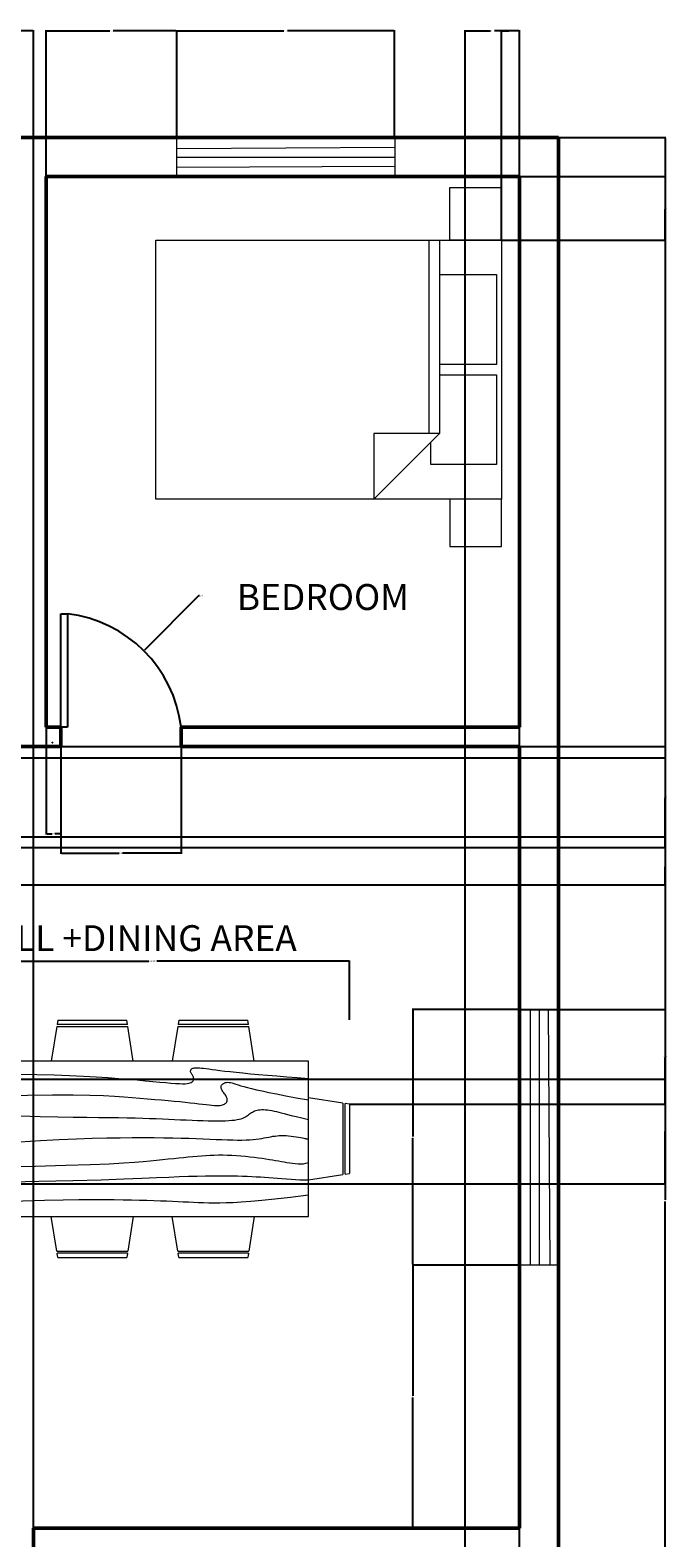
# Model space of a CAD drawing. Units: inches. Extents: x 1926 to 2293, y 1738 to 2280.
# Tile 6 of 6: x 2135 to 2282, y 1931 to 2280. Entities that reach past the tile are written whole.
import ezdxf

# ---------------------------------------------------------------- set-up
doc = ezdxf.new("R2010")
doc.units = ezdxf.units.IN
for name, color, linetype, lineweight in [('A-ANNO-DIMS', 2, 'Continuous', 18), ('A-AREA-IDEN', 7, 'Continuous', 25), ('A-DOOR', 3, 'Continuous', 25), ('A-FURN', 8, 'Continuous', 18), ('A-GLAZ', 4, 'Continuous', 18), ('A-WALL', 7, 'Continuous', 50)]:
    doc.layers.add(name, color=color, linetype=linetype, lineweight=lineweight)
doc.styles.get("Standard").update_dxf_attribs({"font": 'arial.ttf'})
doc.dimstyles.get("Standard").update_dxf_attribs({"dimtxt": 0.18, "dimasz": 0.18, "dimexe": 0.18, "dimexo": 0.0625, "dimgap": 0.09, "dimtad": 0, "dimtih": 1, "dimtoh": 1, "dimdec": 4, "dimzin": 0, "dimdsep": 46, "dimtxsty": 'Standard', "dimcen": 0.09, "dimadec": 0, "dimazin": 0, "dimtfac": 1, "dimtdec": 4, "dimtofl": 0, "dimtmove": 0, "dimatfit": 3, "dimfxl": 1, "dimtolj": 1, "dimtzin": 0, "dimarcsym": 0})

# ---------------------------------------------------------------- blocks, each defined once
blk = doc.blocks.new('Dining Set - 36 x 72 in.')
for p, q in [((-22.2343, 26.00059), (-23.4847, 17.99762)), ((-22.2304, 26), (-5.7608, 26)), ((-22, 27.5), (-22.1562, 26.50042)), ((-5.8416, 26.5), (-22.1534, 26.5)), ((-22, 27.5), (-6, 27.5)), ((-5.8437, 26.49966), (-6, 27.5)), ((-4.5152, 17.99762), (-5.7655, 25.99926)), ((5.7657, 26.00059), (4.5153, 17.99762)), ((5.7696, 26), (22.2392, 26)), ((6, 27.5), (5.8438, 26.50042)), ((22.1584, 26.5), (5.8466, 26.5)), ((6, 27.5), (22, 27.5)), ((22.1563, 26.49966), (22, 27.5)), ((23.4848, 17.99762), (22.2345, 25.99926)), ((36, 18), (-36, 18)), ((-36, 18), (-36, -18)), ((36, -18), (36, 18)), ((-45.5, 8), (-44.5004, 8.15617)), ((-45.5, 8), (-45.5, -8)), ((-44.5, -8.15843), (-44.5, 8.15338)), ((-44.0006, 8.23428), (-35.9976, 9.48474)), ((-44, 8.23041), (-44, -8.23915)), ((44.0006, 8.23428), (35.9976, 9.48474)), ((44, 8.23041), (44, -8.23915)), ((44.5, -8.15843), (44.5, 8.15338)), ((45.5, 8), (44.5005, 8.15617)), ((45.5, 8), (45.5, -8)), ((-44.4997, -8.15631), (-45.5, -8)), ((-35.9976, -9.48476), (-43.9993, -8.2345)), ((35.9976, -9.48476), (43.9993, -8.2345)), ((44.4997, -8.15631), (45.5, -8)), ((-36, -18), (36, -18)), ((-22.2343, -26.0006), (-23.4847, -17.99762)), ((-4.5152, -17.99762), (-5.7655, -25.99928)), ((5.7657, -26.0006), (4.5153, -17.99762)), ((23.4848, -17.99762), (22.2345, -25.99928)), ((-22.2304, -26), (-5.7608, -26)), ((-22, -27.5), (-22.1562, -26.50044)), ((-5.8416, -26.5), (-22.1534, -26.5)), ((-22, -27.5), (-6, -27.5)), ((-5.8437, -26.49967), (-6, -27.5)), ((5.7696, -26), (22.2392, -26)), ((6, -27.5), (5.8438, -26.50044)), ((22.1584, -26.5), (5.8466, -26.5)), ((6, -27.5), (22, -27.5)), ((22.1563, -26.49967), (22, -27.5))]:
    blk.add_line(p, q)
for points in [[(-36, 15), (-31.1772, 14.97754), (-26.8079, 14.91406), (-22.8538, 14.81543), (-19.276, 14.6875), (-16.0362, 14.53613), (-13.0957, 14.36718), (-10.4159, 14.18652), (-7.9583, 14), (-5.6904, 13.81315), (-3.6035, 13.63021), (-1.6954, 13.45508), (0.0365, 13.29166), (1.5945, 13.14388), (2.9811, 13.01562), (4.1988, 12.9108), (5.25, 12.83333), (6.1393, 12.78613), (6.8802, 12.76823), (7.4883, 12.77767), (7.9792, 12.8125), (8.3685, 12.87077), (8.6719, 12.95052), (8.9049, 13.0498), (9.0833, 13.16666), (9.2205, 13.29899), (9.3216, 13.44401), (9.3895, 13.59879), (9.4271, 13.76041), (9.4373, 13.92594), (9.4232, 14.09245), (9.3875, 14.257), (9.3333, 14.41666), (9.2638, 14.56917), (9.1836, 14.71484), (9.0975, 14.85465), (9.0104, 14.98958), (8.9272, 15.1206), (8.8529, 15.2487), (8.7922, 15.37483), (8.75, 15.5), (8.7305, 15.62467), (8.7344, 15.74739), (8.7617, 15.86621), (8.8125, 15.97916), (8.8867, 16.08431), (8.9844, 16.17968), (9.1055, 16.26334), (9.25, 16.33333), (9.4189, 16.38802), (9.6172, 16.42708), (9.8506, 16.45052), (10.125, 16.45833), (10.4463, 16.45052), (10.8203, 16.42708), (11.2529, 16.38802), (11.75, 16.33333), (12.3184, 16.26318), (12.9694, 16.17838), (13.7151, 16.07991), (14.5677, 15.96875), (15.5395, 15.84586), (16.6426, 15.71224), (17.8893, 15.56884), (19.2917, 15.41666), (20.859, 15.25667), (22.5879, 15.08984), (24.4721, 14.91715), (26.5052, 14.73958), (28.6809, 14.5581), (30.9929, 14.3737), (33.4347, 14.18733), (36, 14)], [(-36, 10), (-28.9766, 10.14274), (-23.1725, 10.20442), (-18.4241, 10.19775), (-14.5677, 10.13541), (-11.4399, 10.03011), (-8.877, 9.89453), (-6.7154, 9.74137), (-4.7917, 9.58333), (-2.9698, 9.43082), (-1.2246, 9.28515), (0.4415, 9.14534), (2.026, 9.01041), (3.5266, 8.87939), (4.9408, 8.7513), (6.266, 8.62516), (7.5, 8.5), (8.6411, 8.37549), (9.6914, 8.2539), (10.6538, 8.13818), (11.5312, 8.03125), (12.3267, 7.93603), (13.043, 7.85547), (13.6831, 7.79248), (14.25, 7.75), (14.7471, 7.7303), (15.1797, 7.73307), (15.5537, 7.75732), (15.875, 7.80208), (16.1494, 7.86637), (16.3828, 7.94922), (16.5811, 8.04964), (16.75, 8.16666), (16.8944, 8.29915), (17.0143, 8.44531), (17.1089, 8.60319), (17.1771, 8.77083), (17.218, 8.94629), (17.2305, 9.1276), (17.2137, 9.31282), (17.1667, 9.5), (17.0895, 9.6875), (16.987, 9.875), (16.8649, 10.0625), (16.7292, 10.25), (16.5856, 10.4375), (16.4401, 10.625), (16.2985, 10.8125), (16.1667, 11), (16.05, 11.18733), (15.9518, 11.3737), (15.8752, 11.5581), (15.8229, 11.73958), (15.798, 11.91715), (15.8034, 12.08984), (15.842, 12.25667), (15.9167, 12.41666), (16.0295, 12.56836), (16.1784, 12.70833), (16.3605, 12.83268), (16.5729, 12.9375), (16.8127, 13.01888), (17.0768, 13.07291), (17.3625, 13.0957), (17.6667, 13.08333), (17.9894, 13.03312), (18.3418, 12.94726), (18.7382, 12.82918), (19.1927, 12.68229), (19.7195, 12.51001), (20.3327, 12.31575), (21.0465, 12.10294), (21.875, 11.875), (22.8357, 11.63354), (23.959, 11.37304), (25.2786, 11.08618), (26.8282, 10.76562), (28.6414, 10.40405), (30.752, 9.99414), (33.1936, 9.52856), (36, 9)], [(-36, 5.5), (-30.7157, 5.3348), (-26.069, 5.20963), (-21.9946, 5.11767), (-18.4271, 5.05208), (-15.3009, 5.00602), (-12.5508, 4.97265), (-10.1112, 4.94515), (-7.9167, 4.91666), (-5.909, 4.88167), (-4.0586, 4.83984), (-2.3429, 4.79215), (-0.7396, 4.73958), (0.7739, 4.6831), (2.22, 4.6237), (3.6213, 4.56233), (5, 4.5), (6.373, 4.43782), (7.7344, 4.3776), (9.0723, 4.32129), (10.375, 4.27083), (11.6309, 4.22819), (12.8281, 4.19531), (13.9551, 4.17415), (15, 4.16666), (15.954, 4.17448), (16.819, 4.19791), (17.6001, 4.23698), (18.3021, 4.29166), (18.9299, 4.36198), (19.4883, 4.44791), (19.9823, 4.54948), (20.4167, 4.66666), (20.7969, 4.79899), (21.1302, 4.94401), (21.4245, 5.09879), (21.6875, 5.26041), (21.9271, 5.42594), (22.1511, 5.59245), (22.3672, 5.757), (22.5834, 5.91666), (22.8065, 6.06868), (23.0404, 6.21093), (23.2879, 6.34147), (23.5521, 6.45833), (23.8358, 6.55957), (24.142, 6.64323), (24.4735, 6.70735), (24.8334, 6.75), (25.2235, 6.76969), (25.642, 6.76692), (26.0858, 6.74267), (26.5521, 6.69791), (27.0379, 6.63362), (27.5404, 6.55078), (28.0565, 6.45036), (28.5834, 6.33333), (29.1242, 6.19987), (29.7071, 6.04687), (30.3661, 5.87044), (31.1354, 5.66666), (32.0493, 5.43164), (33.142, 5.16146), (34.4475, 4.85221), (36, 4.5)], [(-36, -1), (-30.7915, -0.6591), (-26.0195, -0.38216), (-21.6519, -0.16284), (-17.6563, 0.00521), (-14.0005, 0.12833), (-10.6523, 0.21289), (-7.5796, 0.26522), (-4.75, 0.29166), (-2.134, 0.29793), (0.2878, 0.28711), (2.5317, 0.26163), (4.6146, 0.22396), (6.5529, 0.17651), (8.3633, 0.12174), (10.0623, 0.06209), (11.6667, 0), (13.1899, -0.06201), (14.6341, -0.1211), (15.9982, -0.17432), (17.2813, -0.21875), (18.4823, -0.25147), (19.6003, -0.26953), (20.6343, -0.27002), (21.5834, -0.25), (22.4481, -0.20768), (23.2357, -0.14584), (23.9549, -0.06836), (24.6146, 0.02083), (25.2235, 0.11784), (25.7904, 0.21875), (26.3241, 0.31966), (26.8334, 0.41666), (27.3265, 0.50618), (27.8099, 0.58593), (28.2894, 0.65397), (28.7709, 0.70833), (29.2601, 0.74707), (29.763, 0.76823), (30.2855, 0.76985), (30.8334, 0.75), (31.4088, 0.70784), (31.9994, 0.64713), (32.589, 0.57275), (33.1615, 0.48958), (33.7008, 0.4025), (34.1908, 0.3164), (34.6153, 0.23616), (34.9584, 0.16666), (35.2099, 0.11165), (35.3848, 0.07031), (35.504, 0.04069), (35.5886, 0.02083), (35.6594, 0.00879), (35.7377, 0.0026), (35.8442, 0.00032), (36, 0)], [(-36, -6.5), (-27.1843, -6.31267), (-20.084, -6.1263), (-14.469, -5.9419), (-10.1094, -5.76042), (-6.7752, -5.58285), (-4.2363, -5.41016), (-2.2629, -5.24333), (-0.625, -5.08334), (0.8708, -4.93099), (2.2715, -4.78646), (3.5872, -4.64974), (4.8281, -4.52084), (6.0046, -4.39974), (7.127, -4.28646), (8.2053, -4.18099), (9.25, -4.08334), (10.2705, -3.99382), (11.2734, -3.91407), (12.2647, -3.84603), (13.25, -3.79167), (14.2354, -3.75293), (15.2266, -3.73177), (16.2295, -3.73015), (17.25, -3.75), (18.2912, -3.79248), (19.3451, -3.85547), (20.4009, -3.93604), (21.4479, -4.03125), (22.4754, -4.13819), (23.4727, -4.25391), (24.4289, -4.37549), (25.3334, -4.5), (26.1785, -4.62492), (26.9694, -4.74935), (27.7145, -4.87281), (28.4219, -4.99479), (29.1, -5.11483), (29.7572, -5.23242), (30.4016, -5.34709), (31.0417, -5.45834), (31.6837, -5.56437), (32.3262, -5.65821), (32.9658, -5.73153), (33.599, -5.77604), (34.2224, -5.78345), (34.8327, -5.74545), (35.4264, -5.65373), (36, -5.5)], [(-36, -10), (-26.4022, -9.81299), (-18.4675, -9.62891), (-11.9839, -9.45069), (-6.7396, -9.28125), (-2.5226, -9.12354), (0.8789, -8.98047), (3.6769, -8.85498), (6.0833, -8.75), (8.2767, -8.66765), (10.3021, -8.60677), (12.1712, -8.56543), (13.8958, -8.54167), (15.4876, -8.53353), (16.9583, -8.53907), (18.3197, -8.55632), (19.5834, -8.58334), (20.7616, -8.61841), (21.8685, -8.66081), (22.9188, -8.71004), (23.9271, -8.76563), (24.9081, -8.82707), (25.8763, -8.89388), (26.8465, -8.96558), (27.8334, -9.04167), (28.8474, -9.12118), (29.8828, -9.20117), (30.93, -9.27824), (31.9792, -9.34896), (33.0205, -9.40991), (34.0443, -9.45768), (35.0407, -9.48885), (36, -9.5)], [(-36, -14.5), (-30.0881, -14.33513), (-25.0332, -14.21224), (-20.7312, -14.12647), (-17.0781, -14.07292), (-13.97, -14.04671), (-11.3027, -14.04297), (-8.9724, -14.05681), (-6.875, -14.08334), (-4.9224, -14.11833), (-3.0905, -14.16016), (-1.3709, -14.20785), (0.2448, -14.26042), (1.7647, -14.3169), (3.1973, -14.3763), (4.5507, -14.43767), (5.8333, -14.5), (7.0554, -14.5621), (8.235, -14.62175), (9.3922, -14.67652), (10.5469, -14.72396), (11.7192, -14.76164), (12.929, -14.78711), (14.1965, -14.79794), (15.5417, -14.79167), (16.9933, -14.76424), (18.6152, -14.70508), (20.4804, -14.60197), (22.6615, -14.44271), (25.2312, -14.21509), (28.2624, -13.9069), (31.8277, -13.50594), (36, -13)]]:
    blk.add_lwpolyline(points)
blk = doc.blocks.new('Bed - Queen')
for p, q in [((0, -80.00003), (0, 0)), ((0, 0), (59.99999, 0)), ((59.99999, 0), (59.99999, -80.00003)), ((7.99999, -1.2), (28.79998, -1.2)), ((7.99999, -14.4), (7.99999, -1.2)), ((28.79998, -1.2), (28.79998, -14.4)), ((31.19999, -1.2), (51.99999, -1.2)), ((31.19999, -14.4), (31.19999, -1.2)), ((51.99999, -1.2), (51.99999, -16.4)), ((0, -14.4), (44.8, -14.4)), ((44.8, -16.8), (0, -16.8)), ((59.99999, -29.6), (44.8, -14.4)), ((44.8, -14.4), (44.8, -29.6)), ((51.99999, -16.4), (46.79936, -16.4)), ((44.8, -29.6), (59.99999, -29.6)), ((59.99999, -80.00003), (0, -80.00003))]:
    blk.add_line(p, q)
blk = doc.blocks.new('*D12')
at = {"layer": 'A-ANNO-DIMS', "color": 0, "lineweight": -2, "transparency": 16777216}
for p, q in [((2117.4, 2050.87), (2117.4, 2064.63)), ((2117.58, 2064.45), (2161.95, 2064.45)), ((2208.22, 2064.45), (2163.85, 2064.45)), ((2208.4, 2050.87), (2208.4, 2064.63))]:
    blk.add_line(p, q, dxfattribs=at)
at = {"layer": 'A-ANNO-DIMS', "color": 0, "transparency": 16777216}
for points in [[(2117.58, 2064.48), (2117.58, 2064.42), (2117.4, 2064.45)], [(2208.22, 2064.48), (2208.22, 2064.42), (2208.4, 2064.45)]]:
    blk.add_solid(points, dxfattribs=at)
at = {"layer": 'Defpoints', "color": 0, "transparency": 16777216}
for p in [(2208.4, 2064.45), (2117.4, 2050.8), (2208.4, 2050.8)]:
    blk.add_point(p, dxfattribs=at)
at = {"layer": 'A-ANNO-DIMS', "color": 0, "transparency": 16777216, "insert": (2162.9, 2064.45), "char_height": 0.18, "attachment_point": 5}
blk.add_mtext('\\A1;DINING SET 91', dxfattribs=at)
blk = doc.blocks.new('*D23')
at = {"layer": 'A-ANNO-DIMS', "color": 0, "lineweight": -2, "transparency": 16777216}
for p, q in [((2138.26, 2246.22), (2138.26, 2280.04)), ((2138.44, 2279.86), (2152.95, 2279.86)), ((2168.25, 2279.86), (2153.74, 2279.86)), ((2168.43, 2255.22), (2168.43, 2280.04))]:
    blk.add_line(p, q, dxfattribs=at)
at = {"layer": 'A-ANNO-DIMS', "color": 0, "transparency": 16777216}
for points in [[(2138.44, 2279.89), (2138.44, 2279.83), (2138.26, 2279.86)], [(2168.25, 2279.89), (2168.25, 2279.83), (2168.43, 2279.86)]]:
    blk.add_solid(points, dxfattribs=at)
at = {"layer": 'Defpoints', "color": 0, "transparency": 16777216}
for p in [(2168.43, 2279.86), (2168.43, 2255.16), (2138.26, 2246.16)]:
    blk.add_point(p, dxfattribs=at)
at = {"layer": 'A-ANNO-DIMS', "color": 0, "transparency": 16777216, "insert": (2153.34, 2279.86), "char_height": 0.18, "attachment_point": 5}
blk.add_mtext('\\A1;30.17', dxfattribs=at)
blk = doc.blocks.new('*D24')
at = {"layer": 'A-ANNO-DIMS', "color": 0, "lineweight": -2, "transparency": 16777216}
for p, q in [((2168.43, 2255.22), (2168.43, 2280.04)), ((2168.61, 2279.86), (2193.25, 2279.86)), ((2218.68, 2279.86), (2194.04, 2279.86)), ((2218.86, 2255.22), (2218.86, 2280.04))]:
    blk.add_line(p, q, dxfattribs=at)
at = {"layer": 'A-ANNO-DIMS', "color": 0, "transparency": 16777216}
for points in [[(2168.61, 2279.89), (2168.61, 2279.83), (2168.43, 2279.86)], [(2218.68, 2279.89), (2218.68, 2279.83), (2218.86, 2279.86)]]:
    blk.add_solid(points, dxfattribs=at)
at = {"layer": 'Defpoints', "color": 0, "transparency": 16777216}
for p in [(2218.86, 2279.86), (2168.43, 2255.16), (2218.86, 2255.16)]:
    blk.add_point(p, dxfattribs=at)
at = {"layer": 'A-ANNO-DIMS', "color": 0, "transparency": 16777216, "insert": (2193.64, 2279.86), "char_height": 0.18, "attachment_point": 5}
blk.add_mtext('\\A1;50.43', dxfattribs=at)
blk = doc.blocks.new('*D44')
at = {"layer": 'A-ANNO-DIMS', "color": 0, "lineweight": -2, "transparency": 16777216}
for p, q in [((2247.69, 1994.08), (2222.88, 1994.08)), ((2223.06, 1993.9), (2223.06, 1963.8)), ((2223.06, 1933.34), (2223.06, 1963.44)), ((2247.69, 1933.16), (2222.88, 1933.16))]:
    blk.add_line(p, q, dxfattribs=at)
at = {"layer": 'A-ANNO-DIMS', "color": 0, "transparency": 16777216}
for points in [[(2223.03, 1993.9), (2223.09, 1993.9), (2223.06, 1994.08)], [(2223.03, 1933.34), (2223.09, 1933.34), (2223.06, 1933.16)]]:
    blk.add_solid(points, dxfattribs=at)
at = {"layer": 'Defpoints', "color": 0, "transparency": 16777216}
for p in [(2223.06, 1994.08), (2247.76, 1994.08), (2247.76, 1933.16)]:
    blk.add_point(p, dxfattribs=at)
at = {"layer": 'A-ANNO-DIMS', "color": 0, "transparency": 16777216, "insert": (2223.06, 1963.62), "char_height": 0.18, "attachment_point": 5}
blk.add_mtext('\\A1;60.92', dxfattribs=at)
blk = doc.blocks.new('*D45')
at = {"layer": 'A-ANNO-DIMS', "color": 0, "lineweight": -2, "transparency": 16777216}
for p, q in [((2247.69, 2053.28), (2222.88, 2053.28)), ((2223.06, 2053.1), (2223.06, 2023.86)), ((2223.06, 1994.26), (2223.06, 2023.5)), ((2247.69, 1994.08), (2222.88, 1994.08))]:
    blk.add_line(p, q, dxfattribs=at)
at = {"layer": 'A-ANNO-DIMS', "color": 0, "transparency": 16777216}
for points in [[(2223.03, 2053.1), (2223.09, 2053.1), (2223.06, 2053.28)], [(2223.03, 1994.26), (2223.09, 1994.26), (2223.06, 1994.08)]]:
    blk.add_solid(points, dxfattribs=at)
at = {"layer": 'Defpoints', "color": 0, "transparency": 16777216}
for p in [(2223.06, 2053.28), (2247.76, 2053.28), (2247.76, 1994.08)]:
    blk.add_point(p, dxfattribs=at)
at = {"layer": 'A-ANNO-DIMS', "color": 0, "transparency": 16777216, "insert": (2223.06, 2023.68), "char_height": 0.18, "attachment_point": 5}
blk.add_mtext('\\A1;59.2', dxfattribs=at)
blk = doc.blocks.new('*D50')
at = {"layer": 'A-ANNO-DIMS', "color": 0, "lineweight": -2, "transparency": 16777216}
for p, q in [((2033.32, 2037.09), (2281.64, 2037.09)), ((2281.46, 2036.91), (2281.46, 2025.19)), ((2281.46, 2013.1), (2281.46, 2024.83)), ((2033.32, 2012.92), (2281.64, 2012.92))]:
    blk.add_line(p, q, dxfattribs=at)
at = {"layer": 'A-ANNO-DIMS', "color": 0, "transparency": 16777216}
for points in [[(2281.43, 2036.91), (2281.49, 2036.91), (2281.46, 2037.09)], [(2281.43, 2013.1), (2281.49, 2013.1), (2281.46, 2012.92)]]:
    blk.add_solid(points, dxfattribs=at)
at = {"layer": 'Defpoints', "color": 0, "transparency": 16777216}
for p in [(2033.26, 2037.09), (2281.46, 2037.09), (2033.26, 2012.92)]:
    blk.add_point(p, dxfattribs=at)
at = {"layer": 'A-ANNO-DIMS', "color": 0, "transparency": 16777216, "insert": (2281.46, 2025.01), "char_height": 0.18, "attachment_point": 5}
blk.add_mtext('\\A1;24.17', dxfattribs=at)
blk = doc.blocks.new('*D52')
at = {"layer": 'A-ANNO-DIMS', "color": 0, "lineweight": -2, "transparency": 16777216}
for p, q in [((2033.32, 2114.16), (2281.64, 2114.16)), ((2281.46, 2113.98), (2281.46, 2102.67)), ((2281.46, 2090.99), (2281.46, 2102.31)), ((2033.32, 2090.81), (2281.64, 2090.81))]:
    blk.add_line(p, q, dxfattribs=at)
at = {"layer": 'A-ANNO-DIMS', "color": 0, "transparency": 16777216}
for points in [[(2281.43, 2113.98), (2281.49, 2113.98), (2281.46, 2114.16)], [(2281.43, 2090.99), (2281.49, 2090.99), (2281.46, 2090.81)]]:
    blk.add_solid(points, dxfattribs=at)
at = {"layer": 'Defpoints', "color": 0, "transparency": 16777216}
for p in [(2033.26, 2114.16), (2281.46, 2114.16), (2033.26, 2090.81)]:
    blk.add_point(p, dxfattribs=at)
at = {"layer": 'A-ANNO-DIMS', "color": 0, "transparency": 16777216, "insert": (2281.46, 2102.49), "char_height": 0.18, "attachment_point": 5}
blk.add_mtext('\\A1;23.348', dxfattribs=at)
blk = doc.blocks.new('*D54')
at = {"layer": 'A-ANNO-DIMS', "color": 0, "lineweight": -2, "transparency": 16777216}
for p, q in [((2021.32, 2111.56), (2281.64, 2111.56)), ((2281.46, 2111.38), (2281.46, 2102.58)), ((2281.46, 2093.41), (2281.46, 2102.21)), ((2021.32, 2093.23), (2281.64, 2093.23))]:
    blk.add_line(p, q, dxfattribs=at)
at = {"layer": 'A-ANNO-DIMS', "color": 0, "transparency": 16777216}
for points in [[(2281.43, 2111.38), (2281.49, 2111.38), (2281.46, 2111.56)], [(2281.43, 2093.41), (2281.49, 2093.41), (2281.46, 2093.23)]]:
    blk.add_solid(points, dxfattribs=at)
at = {"layer": 'Defpoints', "color": 0, "transparency": 16777216}
for p in [(2021.25, 2111.56), (2281.46, 2111.56), (2021.25, 2093.23)]:
    blk.add_point(p, dxfattribs=at)
at = {"layer": 'A-ANNO-DIMS', "color": 0, "transparency": 16777216, "insert": (2281.46, 2102.39), "char_height": 0.18, "attachment_point": 5}
blk.add_mtext('\\A1;18.332', dxfattribs=at)
blk = doc.blocks.new('*D58')
at = {"layer": 'A-ANNO-DIMS', "color": 0, "lineweight": -2, "transparency": 16777216}
for p, q in [((1987.58, 2090.81), (2281.64, 2090.81)), ((2281.46, 2090.63), (2281.46, 2086.66)), ((2281.46, 2082.31), (2281.46, 2086.29)), ((1986.63, 2082.13), (2281.64, 2082.13))]:
    blk.add_line(p, q, dxfattribs=at)
at = {"layer": 'A-ANNO-DIMS', "color": 0, "transparency": 16777216}
for points in [[(2281.43, 2090.63), (2281.49, 2090.63), (2281.46, 2090.81)], [(2281.43, 2082.31), (2281.49, 2082.31), (2281.46, 2082.13)]]:
    blk.add_solid(points, dxfattribs=at)
at = {"layer": 'Defpoints', "color": 0, "transparency": 16777216}
for p in [(1987.52, 2090.81), (2281.46, 2090.81), (1986.57, 2082.13)]:
    blk.add_point(p, dxfattribs=at)
at = {"layer": 'A-ANNO-DIMS', "color": 0, "transparency": 16777216, "insert": (2281.46, 2086.47), "char_height": 0.18, "attachment_point": 5}
blk.add_mtext('\\A1;8.682', dxfattribs=at)
blk = doc.blocks.new('*D61')
at = {"layer": 'A-ANNO-DIMS', "color": 0, "lineweight": -2, "transparency": 16777216}
for p, q in [((2082.76, 1933.22), (2082.76, 2280.04)), ((2082.94, 2279.86), (2108.63, 2279.86)), ((2135.12, 2279.86), (2109.42, 2279.86)), ((2135.3, 1933.22), (2135.3, 2280.04))]:
    blk.add_line(p, q, dxfattribs=at)
at = {"layer": 'A-ANNO-DIMS', "color": 0, "transparency": 16777216}
for points in [[(2082.94, 2279.89), (2082.94, 2279.83), (2082.76, 2279.86)], [(2135.12, 2279.89), (2135.12, 2279.83), (2135.3, 2279.86)]]:
    blk.add_solid(points, dxfattribs=at)
at = {"layer": 'Defpoints', "color": 0, "transparency": 16777216}
for p in [(2135.3, 2279.86), (2082.76, 1933.16), (2135.3, 1933.16)]:
    blk.add_point(p, dxfattribs=at)
at = {"layer": 'A-ANNO-DIMS', "color": 0, "transparency": 16777216, "insert": (2109.03, 2279.86), "char_height": 0.18, "attachment_point": 5}
blk.add_mtext('\\A1;52.54', dxfattribs=at)
blk = doc.blocks.new('*D65')
at = {"layer": 'A-ANNO-DIMS', "color": 0, "lineweight": -2, "transparency": 16777216}
for p, q in [((2141.63, 2114.1), (2141.63, 2089.28)), ((2169.44, 2114.1), (2169.44, 2089.28)), ((2141.81, 2089.46), (2155.15, 2089.46)), ((2169.26, 2089.46), (2155.91, 2089.46))]:
    blk.add_line(p, q, dxfattribs=at)
at = {"layer": 'A-ANNO-DIMS', "color": 0, "transparency": 16777216}
for points in [[(2141.81, 2089.49), (2141.81, 2089.43), (2141.63, 2089.46)], [(2169.26, 2089.49), (2169.26, 2089.43), (2169.44, 2089.46)]]:
    blk.add_solid(points, dxfattribs=at)
at = {"layer": 'Defpoints', "color": 0, "transparency": 16777216}
for p in [(2141.63, 2114.16), (2169.44, 2114.16), (2141.63, 2089.46)]:
    blk.add_point(p, dxfattribs=at)
at = {"layer": 'A-ANNO-DIMS', "color": 0, "transparency": 16777216, "insert": (2155.53, 2089.46), "char_height": 0.18, "attachment_point": 5}
blk.add_mtext('\\A1;27.81', dxfattribs=at)
blk = doc.blocks.new('*D66')
at = {"layer": 'A-ANNO-DIMS', "color": 0, "lineweight": -2, "transparency": 16777216}
for p, q in [((2138.26, 2118.6), (2138.26, 2093.78)), ((2141.63, 2118.6), (2141.63, 2093.78)), ((2138.44, 2093.96), (2139.62, 2093.96)), ((2141.45, 2093.96), (2140.27, 2093.96))]:
    blk.add_line(p, q, dxfattribs=at)
at = {"layer": 'A-ANNO-DIMS', "color": 0, "transparency": 16777216}
for points in [[(2138.44, 2093.99), (2138.44, 2093.93), (2138.26, 2093.96)], [(2141.45, 2093.99), (2141.45, 2093.93), (2141.63, 2093.96)]]:
    blk.add_solid(points, dxfattribs=at)
at = {"layer": 'Defpoints', "color": 0, "transparency": 16777216}
for p in [(2138.26, 2118.66), (2141.63, 2118.66), (2138.26, 2093.96)]:
    blk.add_point(p, dxfattribs=at)
at = {"layer": 'A-ANNO-DIMS', "color": 0, "transparency": 16777216, "insert": (2139.94, 2093.96), "char_height": 0.18, "attachment_point": 5}
blk.add_mtext('\\A1;3.37', dxfattribs=at)
blk = doc.blocks.new('*D72')
at = {"layer": 'A-ANNO-DIMS', "color": 0, "lineweight": -2, "transparency": 16777216}
for p, q in [((2235.21, 1911.29), (2235.21, 2280.04)), ((2235.39, 2279.86), (2241.03, 2279.86)), ((2247.58, 2279.86), (2241.94, 2279.86)), ((2247.76, 1928.72), (2247.76, 2280.04))]:
    blk.add_line(p, q, dxfattribs=at)
at = {"layer": 'A-ANNO-DIMS', "color": 0, "transparency": 16777216}
for points in [[(2235.39, 2279.89), (2235.39, 2279.83), (2235.21, 2279.86)], [(2247.58, 2279.89), (2247.58, 2279.83), (2247.76, 2279.86)]]:
    blk.add_solid(points, dxfattribs=at)
at = {"layer": 'Defpoints', "color": 0, "transparency": 16777216}
for p in [(2247.76, 2279.86), (2247.76, 1928.66), (2235.21, 1911.23)]:
    blk.add_point(p, dxfattribs=at)
at = {"layer": 'A-ANNO-DIMS', "color": 0, "transparency": 16777216, "insert": (2241.48, 2279.86), "char_height": 0.18, "attachment_point": 5}
blk.add_mtext('\\A1;12.546', dxfattribs=at)
blk = doc.blocks.new('*D77')
at = {"layer": 'A-ANNO-DIMS', "color": 0, "lineweight": -2, "transparency": 16777216}
for p, q in [((2243.61, 2231.5), (2243.61, 2280.04)), ((2243.79, 2279.86), (2245.29, 2279.86)), ((2247.58, 2279.86), (2246.08, 2279.86)), ((2247.76, 2246.22), (2247.76, 2280.04))]:
    blk.add_line(p, q, dxfattribs=at)
at = {"layer": 'A-ANNO-DIMS', "color": 0, "transparency": 16777216}
for points in [[(2243.79, 2279.89), (2243.79, 2279.83), (2243.61, 2279.86)], [(2247.58, 2279.89), (2247.58, 2279.83), (2247.76, 2279.86)]]:
    blk.add_solid(points, dxfattribs=at)
at = {"layer": 'Defpoints', "color": 0, "transparency": 16777216}
for p in [(2247.76, 2279.86), (2247.76, 2246.16), (2243.61, 2231.44)]:
    blk.add_point(p, dxfattribs=at)
at = {"layer": 'A-ANNO-DIMS', "color": 0, "transparency": 16777216, "insert": (2245.68, 2279.86), "char_height": 0.18, "attachment_point": 5}
blk.add_mtext('\\A1;4.148', dxfattribs=at)
blk = doc.blocks.new('*D78')
at = {"layer": 'A-ANNO-DIMS', "color": 0, "lineweight": -2, "transparency": 16777216}
for p, q in [((2247.82, 2246.16), (2281.64, 2246.16)), ((2281.46, 2245.98), (2281.46, 2238.98)), ((2281.46, 2231.62), (2281.46, 2238.62)), ((2243.67, 2231.44), (2281.64, 2231.44))]:
    blk.add_line(p, q, dxfattribs=at)
at = {"layer": 'A-ANNO-DIMS', "color": 0, "transparency": 16777216}
for points in [[(2281.43, 2245.98), (2281.49, 2245.98), (2281.46, 2246.16)], [(2281.43, 2231.62), (2281.49, 2231.62), (2281.46, 2231.44)]]:
    blk.add_solid(points, dxfattribs=at)
at = {"layer": 'Defpoints', "color": 0, "transparency": 16777216}
for p in [(2247.76, 2246.16), (2281.46, 2246.16), (2243.61, 2231.44)]:
    blk.add_point(p, dxfattribs=at)
at = {"layer": 'A-ANNO-DIMS', "color": 0, "transparency": 16777216, "insert": (2281.46, 2238.8), "char_height": 0.18, "attachment_point": 5}
blk.add_mtext('\\A1;14.727', dxfattribs=at)
blk = doc.blocks.new('*D82')
at = {"layer": 'A-ANNO-DIMS', "color": 0, "lineweight": -2, "transparency": 16777216}
for p, q in [((2247.82, 2053.28), (2281.64, 2053.28)), ((2281.46, 2053.1), (2281.46, 2042.47)), ((2281.46, 2031.48), (2281.46, 2042.11)), ((2208.46, 2031.3), (2281.64, 2031.3))]:
    blk.add_line(p, q, dxfattribs=at)
at = {"layer": 'A-ANNO-DIMS', "color": 0, "transparency": 16777216}
for points in [[(2281.43, 2053.1), (2281.49, 2053.1), (2281.46, 2053.28)], [(2281.43, 2031.48), (2281.49, 2031.48), (2281.46, 2031.3)]]:
    blk.add_solid(points, dxfattribs=at)
at = {"layer": 'Defpoints', "color": 0, "transparency": 16777216}
for p in [(2247.76, 2053.28), (2281.46, 2053.28), (2208.4, 2031.3)]:
    blk.add_point(p, dxfattribs=at)
at = {"layer": 'A-ANNO-DIMS', "color": 0, "transparency": 16777216, "insert": (2281.46, 2042.29), "char_height": 0.18, "attachment_point": 5}
blk.add_mtext('\\A1;21.975', dxfattribs=at)
blk = doc.blocks.new('*D86')
at = {"layer": 'A-ANNO-DIMS', "color": 0, "lineweight": -2, "transparency": 16777216}
for p, q in [((2256.82, 2255.16), (2281.64, 2255.16)), ((2281.46, 2254.98), (2281.46, 2009.19)), ((2281.46, 1763.03), (2281.46, 2008.83)), ((2141.98, 1762.85), (2281.64, 1762.85))]:
    blk.add_line(p, q, dxfattribs=at)
at = {"layer": 'A-ANNO-DIMS', "color": 0, "transparency": 16777216}
for points in [[(2281.43, 2254.98), (2281.49, 2254.98), (2281.46, 2255.16)], [(2281.43, 1763.03), (2281.49, 1763.03), (2281.46, 1762.85)]]:
    blk.add_solid(points, dxfattribs=at)
at = {"layer": 'Defpoints', "color": 0, "transparency": 16777216}
for p in [(2256.76, 2255.16), (2281.46, 2255.16), (2141.91, 1762.85)]:
    blk.add_point(p, dxfattribs=at)
at = {"layer": 'A-ANNO-DIMS', "color": 0, "transparency": 16777216, "insert": (2281.46, 2009.01), "char_height": 0.18, "attachment_point": 5}
blk.add_mtext('\\A1;492.3', dxfattribs=at)
blk = doc.blocks.new('*D89')
at = {"layer": 'A-ANNO-DIMS', "color": 0, "lineweight": -2, "transparency": 16777216}
for p, q in [((2173.51, 2149.06), (2160.96, 2136.46)), ((2173.69, 2149.06), (2173.51, 2149.06)), ((2139.61, 2115.11), (2139.79, 2115.11)), ((2139.7, 2115.02), (2139.7, 2115.2))]:
    blk.add_line(p, q, dxfattribs=at)
at = {"layer": 'A-ANNO-DIMS', "color": 0, "transparency": 16777216}
blk.add_solid([(2160.94, 2136.48), (2160.98, 2136.44), (2160.83, 2136.33)], dxfattribs=at)
at = {"layer": 'Defpoints', "color": 0, "transparency": 16777216}
for p in [(2160.83, 2136.33), (2139.7, 2115.11)]:
    blk.add_point(p, dxfattribs=at)
at = {"layer": 'A-ANNO-DIMS', "color": 0, "transparency": 16777216, "insert": (2174.18, 2149.06), "char_height": 0.18, "attachment_point": 5}
blk.add_mtext('\\A1;R29.95', dxfattribs=at)

msp = doc.modelspace()

# ---------------------------------------------------------------- linework, layer by layer
at = {"layer": 'A-DOOR'}
for p, q in [((2141.6268, 2118.6622), (2141.6268, 2144.8627)), ((2141.6268, 2144.8627), (2143.1305, 2144.8627)), ((2143.1305, 2144.8627), (2143.1305, 2118.6622)), ((2143.1305, 2118.6622), (2141.6268, 2118.6622))]:
    msp.add_line(p, q, dxfattribs=at)
msp.add_arc((2139.696, 2115.1086), 29.9517, 6.813989, 83.415495, dxfattribs=at)
at = {"layer": 'A-FURN'}
for points in [[(2243.6086, 2231.4351), (2231.6086, 2231.4351), (2231.6086, 2243.6337), (2243.6086, 2243.6337)], [(2243.6086, 2171.4351), (2231.6086, 2171.4351), (2231.6086, 2160.4664), (2243.6086, 2160.4664)]]:
    msp.add_lwpolyline(points, close=True, dxfattribs=at)
at = {"layer": 'A-GLAZ'}
for p, q in [((2168.4281, 2252.6703), (2218.8619, 2252.9679)), ((2168.4281, 2250.6622), (2218.8619, 2250.6622)), ((2168.4281, 2248.2834), (2218.8619, 2248.5131)), ((2250.1899, 2053.2792), (2250.1899, 1994.0776)), ((2252.2569, 2053.2792), (2252.2569, 1994.0776)), ((2254.3822, 2053.2792), (2254.7548, 1994.0776))]:
    msp.add_line(p, q, dxfattribs=at)
for points in [[(2168.4281, 2255.1622), (2218.8619, 2255.1622), (2218.8619, 2246.1622), (2168.4281, 2246.1622)], [(2247.7569, 2053.2792), (2256.7569, 2053.2792), (2256.7569, 1994.0776), (2247.7569, 1994.0776)]]:
    msp.add_lwpolyline(points, close=True, dxfattribs=at)
at = {"layer": 'A-WALL'}
for p, q in [((1950.7569, 2255.1622), (2256.7569, 2255.1622)), ((2256.7569, 2255.1622), (2256.7569, 1793.1622)), ((2138.2569, 2118.6622), (2138.2569, 2246.1622)), ((2138.2569, 2246.1622), (2247.7569, 2246.1622)), ((2247.7569, 2246.1622), (2247.7569, 2118.6622)), ((2138.2569, 2118.6622), (2141.6268, 2118.6622)), ((2141.6268, 2114.1622), (2141.6268, 2118.6622)), ((2169.4361, 2114.1622), (2169.4361, 2118.6622)), ((2169.4361, 2118.6622), (2247.7569, 2118.6622)), ((2103.7569, 2114.1622), (2141.6268, 2114.1622)), ((2169.4361, 2114.1622), (2247.7569, 2114.1622)), ((2247.7569, 2114.1622), (2247.7569, 1933.1622)), ((2247.7569, 1933.1622), (2135.2979, 1933.1622)), ((2135.2979, 1928.6622), (2135.2979, 1933.1622))]:
    msp.add_line(p, q, dxfattribs=at)

# ---------------------------------------------------------------- block references
at = {"layer": 'A-FURN', "rotation": 270}
msp.add_blockref('Bed - Queen', (2243.6086, 2231.4351), dxfattribs=at)
at = {"layer": 'A-FURN'}
msp.add_blockref('Dining Set - 36 x 72 in.', (2162.8994, 2023.3046), dxfattribs=at)

# ---------------------------------------------------------------- texts
at = {"layer": 'A-AREA-IDEN', "char_height": 6, "attachment_point": 1}
for s, width, insert in [('BEDROOM', 23.953264, (2182.349, 2151.7759)), ('HALL +DINING AREA', 89.283239, (2120.3037, 2072.7791))]:
    msp.add_mtext_dynamic_manual_height_columns(s, width=width, gutter_width=12.5, heights=[0], dxfattribs=dict(at, insert=insert))

# ---------------------------------------------------------------- dimensions: what is measured, and where the dimension line sits
at = {"layer": 'A-ANNO-DIMS'}
for base, p1, p2, override, picture, middle in [((2135.2979, 2279.8622), (2082.7569, 1933.1622), (2135.2979, 1933.1622), {"dimdec": 2, "dimlfac": 1, "dimrnd": 0, "dimzin": 0, "dimdsep": 46, "dimlunit": 2}, '*D61', (2109.0274, 2279.8622)), ((2168.4281, 2279.8622), (2138.2569, 2246.1622), (2168.4281, 2255.1622), {"dimdec": 2, "dimlfac": 1, "dimrnd": 0, "dimzin": 0, "dimdsep": 46, "dimlunit": 2}, '*D23', (2153.3425, 2279.8622)), ((2218.8619, 2279.8622), (2168.4281, 2255.1622), (2218.8619, 2255.1622), {"dimdec": 2, "dimlfac": 1, "dimrnd": 0, "dimzin": 0, "dimdsep": 46, "dimlunit": 2}, '*D24', (2193.645, 2279.8622)), ((2247.7569, 2279.8622), (2235.2111, 1911.2306), (2247.7569, 1928.6622), {"dimdec": 3, "dimlfac": 1, "dimrnd": 0, "dimzin": 0, "dimdsep": 46, "dimlunit": 2}, '*D72', (2241.484, 2279.8622)), ((2247.7569, 2279.8622), (2243.6086, 2231.4351), (2247.7569, 2246.1622), {"dimdec": 3, "dimlfac": 1, "dimrnd": 0, "dimzin": 0, "dimdsep": 46, "dimlunit": 2}, '*D77', (2245.6827, 2279.8622))]:
    dim = msp.add_linear_dim(base=base, p1=p1, p2=p2, dimstyle='Standard', override=override, dxfattribs=at)
    dim.commit()
    dim.dimension.update_dxf_attribs({"geometry": picture, "text_midpoint": middle})
for base, p1, p2, angle, override, picture, middle in [((2281.4569, 2255.1622), (2141.9148, 1762.8524), (2256.7569, 2255.1622), 90, {"dimdec": 1, "dimlfac": 1, "dimrnd": 0, "dimzin": 0, "dimdsep": 46, "dimlunit": 2}, '*D86', (2281.4569, 2009.0073)), ((2281.4569, 2246.1622), (2243.6086, 2231.4351), (2247.7569, 2246.1622), 90, {"dimdec": 3, "dimlfac": 1, "dimrnd": 0, "dimzin": 0, "dimdsep": 46, "dimlunit": 2}, '*D78', (2281.4569, 2238.7987)), ((2138.2569, 2093.9622), (2141.6268, 2118.6622), (2138.2569, 2118.6622), 180, {"dimdec": 2, "dimlfac": 1, "dimrnd": 0, "dimzin": 0, "dimdsep": 46, "dimlunit": 2}, '*D66', (2139.9418, 2093.9622)), ((2281.4569, 2114.1622), (2033.2569, 2090.8146), (2033.2569, 2114.1622), 90, {"dimdec": 3, "dimlfac": 1, "dimrnd": 0, "dimzin": 0, "dimdsep": 46, "dimlunit": 2}, '*D52', (2281.4569, 2102.4884)), ((2141.6268, 2089.4622), (2169.4361, 2114.1622), (2141.6268, 2114.1622), 180, {"dimdec": 2, "dimlfac": 1, "dimrnd": 0, "dimzin": 0, "dimdsep": 46, "dimlunit": 2}, '*D65', (2155.5314, 2089.4622)), ((2281.4569, 2111.5596), (2021.2546, 2093.2275), (2021.2546, 2111.5596), 90, {"dimdec": 3, "dimlfac": 1, "dimrnd": 0, "dimzin": 0, "dimdsep": 46, "dimlunit": 2}, '*D54', (2281.4569, 2102.3935)), ((2281.4569, 2090.8146), (1986.5655, 2082.133), (1987.5186, 2090.8146), 90, {"dimdec": 3, "dimlfac": 1, "dimrnd": 0, "dimzin": 0, "dimdsep": 46, "dimlunit": 2}, '*D58', (2281.4569, 2086.4738)), ((2281.4569, 2053.2792), (2208.3994, 2031.3046), (2247.7569, 2053.2792), 90, {"dimdec": 3, "dimlfac": 1, "dimrnd": 0, "dimzin": 0, "dimdsep": 46, "dimlunit": 2}, '*D82', (2281.4569, 2042.2919)), ((2223.0569, 2053.2792), (2247.7569, 1994.0776), (2247.7569, 2053.2792), 90, {"dimdec": 1, "dimlfac": 1, "dimrnd": 0, "dimzin": 0, "dimdsep": 46, "dimlunit": 2}, '*D45', (2223.0569, 2023.6784)), ((2281.4569, 2037.0927), (2033.2569, 2012.9217), (2033.2569, 2037.0927), 90, {"dimdec": 2, "dimlfac": 1, "dimrnd": 0, "dimzin": 0, "dimdsep": 46, "dimlunit": 2}, '*D50', (2281.4569, 2025.0072)), ((2223.0569, 1994.0776), (2247.7569, 1933.1622), (2247.7569, 1994.0776), 90, {"dimdec": 2, "dimlfac": 1, "dimrnd": 0, "dimzin": 0, "dimdsep": 46, "dimlunit": 2}, '*D44', (2223.0569, 1963.6199))]:
    dim = msp.add_linear_dim(base=base, p1=p1, p2=p2, angle=angle, dimstyle='Standard', override=override, dxfattribs=at)
    dim.commit()
    dim.dimension.update_dxf_attribs({"geometry": picture, "text_midpoint": middle})
dim = msp.add_radius_dim(center=(2139.696, 2115.1086), mpoint=(2160.8328, 2136.3298), dimstyle='Standard', override={"dimdec": 2, "dimlfac": 1, "dimrnd": 0, "dimzin": 0, "dimdsep": 46, "dimlunit": 2}, dxfattribs=at)
dim.commit()
dim.dimension.update_dxf_attribs({"geometry": '*D89', "text_midpoint": (2174.1754, 2149.0625), "dimtype": 164})
dim = msp.add_linear_dim(base=(2208.3994, 2064.4546), p1=(2117.3994, 2050.8046), p2=(2208.3994, 2050.8046), text='DINING SET <>', dimstyle='Standard', override={"dimdec": 0, "dimlfac": 1, "dimrnd": 0, "dimzin": 0, "dimdsep": 46, "dimlunit": 2}, dxfattribs=at)
dim.commit()
dim.dimension.update_dxf_attribs({"geometry": '*D12', "text_midpoint": (2162.8994, 2064.4546)})

doc.saveas('drawing.dxf')
